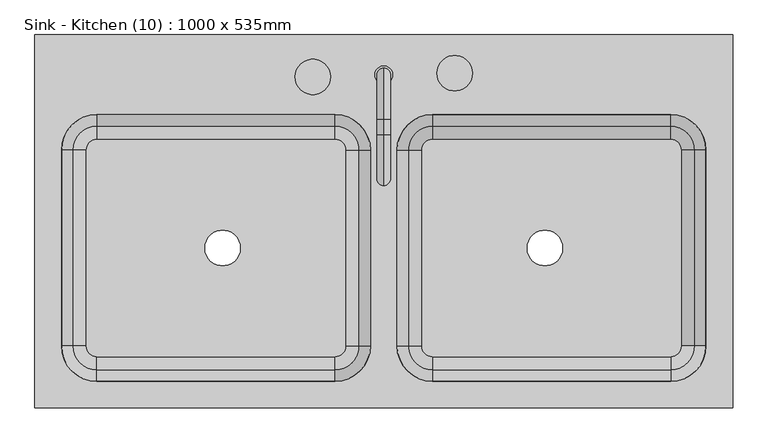
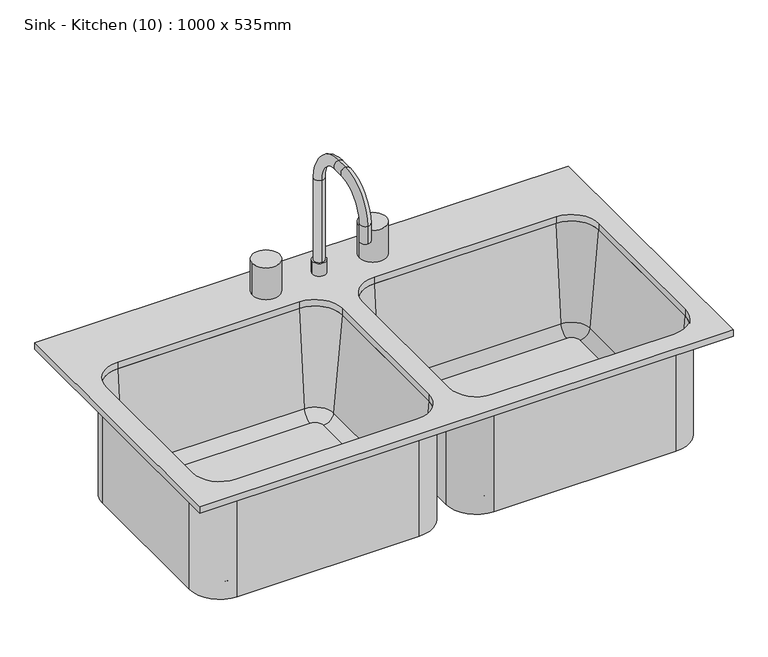
"""IFC4 building model written with IfcOpenShell, lengths in millimetres: flow terminal geometry, Sink - Kitchen (10) : 1000 x 535mm."""

from ifc_helpers import new_model, si_unit, point, frame, frame_2d, origin, place, context, project, spatial, polyline, circle_curve, ellipse_curve, trimmed, segment, composite_curve, outline, extrude, source, transform, mapped, element, save
from ifc_brep_helpers import plane_surface, cylinder_surface, revolved_surface, advanced_brep


def sink_kitchen_10_1000_x_535mm_bc591ed5(model_context):
    return source(origin(), model_context, "Body", "SolidModel", [
        extrude(outline(polyline([(515.6892406, 269.8454011), (515.6892406, -265.1545989), (-484.3107594, -265.1545989), (-484.3107594, 269.8454011), (515.6892406, 269.8454011)]), holes=[composite_curve([segment(polyline([(-54.1607594, 155.5454011), (-395.4107594, 155.5454011)]), True, "CONTINUOUS"), segment(trimmed(circle_curve(frame_2d((-395.4107594, 104.7454011)), 50.8), [point((-395.4107594, 155.5454011))], [point((-446.2107594, 104.7454011))], True, "CARTESIAN"), True, "CONTINUOUS"), segment(polyline([(-446.2107594, 104.7454011), (-446.2107594, -176.2545989)]), True, "CONTINUOUS"), segment(trimmed(circle_curve(frame_2d((-395.4107594, -176.2545989)), 50.8), [point((-446.2107594, -176.2545989))], [point((-395.4107594, -227.0545989))], True, "CARTESIAN"), True, "CONTINUOUS"), segment(polyline([(-395.4107594, -227.0545989), (-54.1607594, -227.0545989)]), True, "CONTINUOUS"), segment(trimmed(circle_curve(frame_2d((-54.1607594, -176.2545989)), 50.8), [point((-54.1607594, -227.0545989))], [point((-3.3607594, -176.2545989))], True, "CARTESIAN"), True, "CONTINUOUS"), segment(polyline([(-3.3607594, -176.2545989), (-3.3607594, 104.7454011)]), True, "CONTINUOUS"), segment(trimmed(circle_curve(frame_2d((-54.1607594, 104.7454011)), 50.8), [point((-3.3607594, 104.7454011))], [point((-54.1607594, 155.5454011))], True, "CARTESIAN"), True, "CONTINUOUS")], self_intersect=False), composite_curve([segment(polyline([(85.5392406, -227.0545989), (426.7892406, -227.0545989)]), True, "CONTINUOUS"), segment(trimmed(circle_curve(frame_2d((426.7892406, -176.2545989)), 50.8), [point((426.7892406, -227.0545989))], [point((477.5892406, -176.2545989))], True, "CARTESIAN"), True, "CONTINUOUS"), segment(polyline([(477.5892406, -176.2545989), (477.5892406, 104.7454011)]), True, "CONTINUOUS"), segment(trimmed(circle_curve(frame_2d((426.7892406, 104.7454011)), 50.8), [point((477.5892406, 104.7454011))], [point((426.7892406, 155.5454011))], True, "CARTESIAN"), True, "CONTINUOUS"), segment(polyline([(426.7892406, 155.5454011), (85.5392406, 155.5454011)]), True, "CONTINUOUS"), segment(trimmed(circle_curve(frame_2d((85.5392406, 104.7454011)), 50.8), [point((85.5392406, 155.5454011))], [point((34.7392406, 104.7454011))], True, "CARTESIAN"), True, "CONTINUOUS"), segment(polyline([(34.7392406, 104.7454011), (34.7392406, -176.2545989)]), True, "CONTINUOUS"), segment(trimmed(circle_curve(frame_2d((85.5392406, -176.2545989)), 50.8), [point((34.7392406, -176.2545989))], [point((85.5392406, -227.0545989))], True, "CARTESIAN"), True, "CONTINUOUS")], self_intersect=False)]), frame((0.0, 0.0, 900.0), z_axis=(0.0, 0.0, 1.0), x_axis=(1.0, 0.0, 0.0)), (0.0, 0.0, 1.0), 12.7),
        extrude(outline(composite_curve([segment(trimmed(circle_curve(frame_2d((-85.9107594, 209.6166076)), 25.4), [point((-111.3107594, 209.6166076))], [point((-60.5107594, 209.6166076))], False, "CARTESIAN"), True, "CONTINUOUS"), segment(trimmed(circle_curve(frame_2d((-85.9107594, 209.6166076)), 25.4), [point((-60.5107594, 209.6166076))], [point((-111.3107594, 209.6166076))], False, "CARTESIAN"), True, "CONTINUOUS")], self_intersect=False)), frame((0.0, 0.0, 912.7), z_axis=(0.0, 0.0, 1.0), x_axis=(1.0, 0.0, 0.0)), (0.0, 0.0, 1.0), 63.5),
        extrude(outline(composite_curve([segment(trimmed(circle_curve(frame_2d((117.2892406, 214.8133323)), 25.4), [point((91.8892406, 214.8133323))], [point((142.6892406, 214.8133323))], False, "CARTESIAN"), True, "CONTINUOUS"), segment(trimmed(circle_curve(frame_2d((117.2892406, 214.8133323)), 25.4), [point((142.6892406, 214.8133323))], [point((91.8892406, 214.8133323))], False, "CARTESIAN"), True, "CONTINUOUS")], self_intersect=False)), frame((0.0, 0.0, 912.7), z_axis=(0.0, 0.0, 1.0), x_axis=(1.0, 0.0, 0.0)), (0.0, 0.0, 1.0), 63.5),
        advanced_brep(
        [(2.9892406, 212.6954011, 912.7), (28.3892406, 212.6954011, 912.7), (15.6892406, 222.2204011, 1100.025), (15.6892406, 203.1704011, 1100.025), (15.6892406, 203.1704011, 938.1), (15.6892406, 222.2204011, 938.1), (15.6892406, 149.1954011, 1173.05), (15.6892406, 149.1954011, 1154.0), (15.6892406, 126.9704011, 1173.05), (15.6892406, 126.9704011, 1154.0), (15.6892406, 53.9454011, 1100.025), (15.6892406, 72.9954011, 1100.025), (15.6892406, 53.9454011, 1065.1), (15.6892406, 72.9954011, 1065.1), (2.9892406, 212.6954011, 938.1), (28.3892406, 212.6954011, 938.1)],
        [
            (0, 1, circle_curve(frame((15.6892406, 212.6954011, 912.7), z_axis=(0.0, 0.0, -1.0), x_axis=(1.0, 0.0, 0.0)), 12.7)),
            (1, 0, circle_curve(frame((15.6892406, 212.6954011, 912.7), z_axis=(0.0, 0.0, -1.0), x_axis=(1.0, 0.0, 0.0)), 12.7)),
            (2, 3, circle_curve(frame((15.6892406, 212.6954011, 1100.025), z_axis=(0.0, 0.0, -1.0), x_axis=(0.0, -1.0, 0.0)), 9.525)),
            (3, 4),
            (4, 5, circle_curve(frame((15.6892406, 212.6954011, 938.1), z_axis=(0.0, 0.0, 1.0), x_axis=(0.0, -1.0, 0.0)), 9.525)),
            (5, 2),
            (3, 2, circle_curve(frame((15.6892406, 212.6954011, 1100.025), z_axis=(0.0, 0.0, -1.0), x_axis=(0.0, -1.0, 0.0)), 9.525)),
            (5, 4, circle_curve(frame((15.6892406, 212.6954011, 938.1), z_axis=(0.0, 0.0, 1.0), x_axis=(0.0, -1.0, 0.0)), 9.525)),
            (2, 6, circle_curve(frame((15.6892406, 149.1954011, 1100.025), z_axis=(1.0, 0.0, 0.0), x_axis=(0.0, 1.0, 0.0)), 73.025)),
            (6, 7, circle_curve(frame((15.6892406, 149.1954011, 1163.525), z_axis=(0.0, 1.0, 0.0), x_axis=(0.0, 0.0, -1.0)), 9.525)),
            (7, 3, circle_curve(frame((15.6892406, 149.1954011, 1100.025), z_axis=(-1.0, 0.0, 0.0), x_axis=(0.0, 1.0, 0.0)), 53.975)),
            (7, 6, circle_curve(frame((15.6892406, 149.1954011, 1163.525), z_axis=(0.0, 1.0, 0.0), x_axis=(0.0, 0.0, -1.0)), 9.525)),
            (6, 8),
            (8, 9, circle_curve(frame((15.6892406, 126.9704011, 1163.525), z_axis=(0.0, 1.0, 0.0), x_axis=(0.0, 0.0, -1.0)), 9.525)),
            (9, 7),
            (9, 8, circle_curve(frame((15.6892406, 126.9704011, 1163.525), z_axis=(0.0, 1.0, 0.0), x_axis=(0.0, 0.0, -1.0)), 9.525)),
            (8, 10, circle_curve(frame((15.6892406, 126.9704011, 1100.025), z_axis=(1.0, 0.0, 0.0), x_axis=(0.0, 0.0, 1.0)), 73.025)),
            (10, 11, circle_curve(frame((15.6892406, 63.4704011, 1100.025), z_axis=(0.0, 0.0, 1.0), x_axis=(0.0, 1.0, 0.0)), 9.525)),
            (11, 9, circle_curve(frame((15.6892406, 126.9704011, 1100.025), z_axis=(-1.0, 0.0, 0.0), x_axis=(0.0, 0.0, 1.0)), 53.975)),
            (11, 10, circle_curve(frame((15.6892406, 63.4704011, 1100.025), z_axis=(0.0, 0.0, 1.0), x_axis=(0.0, 1.0, 0.0)), 9.525)),
            (12, 13, circle_curve(frame((15.6892406, 63.4704011, 1065.1), z_axis=(0.0, 0.0, -1.0), x_axis=(0.0, 1.0, 0.0)), 9.525)),
            (13, 12, circle_curve(frame((15.6892406, 63.4704011, 1065.1), z_axis=(0.0, 0.0, -1.0), x_axis=(0.0, 1.0, 0.0)), 9.525)),
            (10, 12),
            (13, 11),
            (14, 15, circle_curve(frame((15.6892406, 212.6954011, 938.1), z_axis=(0.0, 0.0, 1.0), x_axis=(1.0, 0.0, 0.0)), 12.7)),
            (15, 14, circle_curve(frame((15.6892406, 212.6954011, 938.1), z_axis=(0.0, 0.0, 1.0), x_axis=(1.0, 0.0, 0.0)), 12.7)),
            (14, 0),
            (1, 15),
        ],
        [
            plane_surface(frame((15.6892406, 203.1704011, 912.7), z_axis=(0.0, 0.0, -1.0), x_axis=(1.0, 0.0, 0.0))),
            cylinder_surface(frame((15.6892406, 212.6954011, 912.7), z_axis=(0.0, 0.0, -1.0), x_axis=(0.0, -1.0, 0.0)), 9.525),
            revolved_surface(trimmed(ellipse_curve(frame((15.6892406, 212.6954011, 1100.025), z_axis=(0.0, 0.0, -1.0), x_axis=(0.0, -1.0, 0.0)), 9.525, 9.525), [point((15.6892406, 222.2204011, 1100.025))], [point((15.6892406, 203.1704011, 1100.025))], True, "CARTESIAN"), (15.6892406, 149.1954011, 1100.025), (1.0, 0.0, 0.0)),
            revolved_surface(trimmed(ellipse_curve(frame((15.6892406, 212.6954011, 1100.025), z_axis=(0.0, 0.0, -1.0), x_axis=(0.0, -1.0, 0.0)), 9.525, 9.525), [point((15.6892406, 203.1704011, 1100.025))], [point((15.6892406, 222.2204011, 1100.025))], True, "CARTESIAN"), (15.6892406, 149.1954011, 1100.025), (1.0, 0.0, 0.0)),
            cylinder_surface(frame((15.6892406, 149.1954011, 1163.525), z_axis=(0.0, 1.0, 0.0), x_axis=(0.0, 0.0, -1.0)), 9.525),
            revolved_surface(trimmed(ellipse_curve(frame((15.6892406, 126.9704011, 1163.525), z_axis=(0.0, 1.0, 0.0), x_axis=(0.0, 0.0, -1.0)), 9.525, 9.525), [point((15.6892406, 126.9704011, 1173.05))], [point((15.6892406, 126.9704011, 1154.0))], True, "CARTESIAN"), (15.6892406, 126.9704011, 1100.025), (1.0, 0.0, 0.0)),
            revolved_surface(trimmed(ellipse_curve(frame((15.6892406, 126.9704011, 1163.525), z_axis=(0.0, 1.0, 0.0), x_axis=(0.0, 0.0, -1.0)), 9.525, 9.525), [point((15.6892406, 126.9704011, 1154.0))], [point((15.6892406, 126.9704011, 1173.05))], True, "CARTESIAN"), (15.6892406, 126.9704011, 1100.025), (1.0, 0.0, 0.0)),
            plane_surface(frame((15.6892406, 53.9454011, 1065.1), z_axis=(0.0, 0.0, -1.0), x_axis=(-1.0, 0.0, 0.0))),
            cylinder_surface(frame((15.6892406, 63.4704011, 1100.025), z_axis=(0.0, 0.0, 1.0), x_axis=(0.0, 1.0, 0.0)), 9.525),
            plane_surface(frame((28.3892406, 212.6954011, 938.1), z_axis=(0.0, 0.0, 1.0), x_axis=(0.0, 1.0, 0.0))),
            cylinder_surface(frame((15.6892406, 212.6954011, 912.7), z_axis=(0.0, 0.0, 1.0), x_axis=(1.0, 0.0, 0.0)), 12.7),
        ],
        [
            (0, [[1, 2]]),
            (1, [[3, 4, 5, 6]]),
            (1, [[7, -6, 8, -4]]),
            (2, [[-3, 9, 10, 11]]),
            (3, [[-7, -11, 12, -9]]),
            (4, [[-10, 13, 14, 15]]),
            (4, [[-12, -15, 16, -13]]),
            (5, [[-14, 17, 18, 19]]),
            (6, [[-16, -19, 20, -17]]),
            (7, [[21, 22]]),
            (8, [[-18, 23, -22, 24]]),
            (8, [[-20, -24, -21, -23]]),
            (9, [[25, 26], [-5, -8]]),
            (10, [[-25, 27, -2, 28]]),
            (10, [[-26, -28, -1, -27]]),
        ],
    ),
        advanced_brep(
        [(-38.8723412, 104.7454011, 693.625), (-54.1607594, 120.0338193, 693.625), (-395.4107594, 120.0338193, 693.625), (-410.6991776, 104.7454011, 693.625), (-410.6991776, -176.2545989, 693.625), (-395.4107594, -191.5430171, 693.625), (-54.1607594, -191.5430171, 693.625), (-38.8723412, -176.2545989, 693.625), (-240.6607594, -35.7545989, 693.625), (-189.8607594, -35.7545989, 693.625), (-452.5607594, 104.7454011, 684.1), (-395.4107594, 161.8954011, 684.1), (-54.1607594, 161.8954011, 684.1), (2.9892406, 104.7454011, 684.1), (2.9892406, -176.2545989, 684.1), (-54.1607594, -233.4045989, 684.1), (-395.4107594, -233.4045989, 684.1), (-452.5607594, -176.2545989, 684.1), (-240.6607594, -35.7545989, 684.1), (-189.8607594, -35.7545989, 684.1), (-54.1607594, 161.8954011, 900.0), (2.9892406, 104.7454011, 900.0), (-19.8948322, 104.7454011, 711.0146831), (-54.1607594, 139.0113283, 711.0146831), (-3.3607594, 104.7454011, 900.0), (-54.1607594, 155.5454011, 900.0), (2.9892406, -176.2545989, 900.0), (-19.8948322, -176.2545989, 711.0146831), (-3.3607594, -176.2545989, 900.0), (-54.1607594, -233.4045989, 900.0), (-54.1607594, -210.5205261, 711.0146831), (-54.1607594, -227.0545989, 900.0), (-395.4107594, -233.4045989, 900.0), (-395.4107594, -210.5205261, 711.0146831), (-395.4107594, -227.0545989, 900.0), (-452.5607594, -176.2545989, 900.0), (-429.6766866, -176.2545989, 711.0146831), (-446.2107594, -176.2545989, 900.0), (-452.5607594, 104.7454011, 900.0), (-429.6766866, 104.7454011, 711.0146831), (-446.2107594, 104.7454011, 900.0), (-395.4107594, 161.8954011, 900.0), (-395.4107594, 139.0113283, 711.0146831), (-395.4107594, 155.5454011, 900.0)],
        [
            (0, 1, circle_curve(frame((-54.1607594, 104.7454011, 693.625), z_axis=(0.0, 0.0, 1.0), x_axis=(0.0, 1.0, 0.0)), 15.2884182)),
            (1, 2),
            (2, 3, circle_curve(frame((-395.4107594, 104.7454011, 693.625), z_axis=(0.0, 0.0, 1.0), x_axis=(-1.0, 0.0, 0.0)), 15.2884182)),
            (3, 4),
            (4, 5, circle_curve(frame((-395.4107594, -176.2545989, 693.625), z_axis=(0.0, 0.0, 1.0), x_axis=(0.0, -1.0, 0.0)), 15.2884182)),
            (5, 6),
            (6, 7, circle_curve(frame((-54.1607594, -176.2545989, 693.625), z_axis=(0.0, 0.0, 1.0), x_axis=(1.0, 0.0, 0.0)), 15.2884182)),
            (7, 0),
            (8, 9, circle_curve(frame((-215.2607594, -35.7545989, 693.625), z_axis=(0.0, 0.0, -1.0), x_axis=(1.0, 0.0, 0.0)), 25.4)),
            (9, 8, circle_curve(frame((-215.2607594, -35.7545989, 693.625), z_axis=(0.0, 0.0, -1.0), x_axis=(1.0, 0.0, 0.0)), 25.4)),
            (10, 11, circle_curve(frame((-395.4107594, 104.7454011, 684.1), z_axis=(0.0, 0.0, -1.0), x_axis=(-1.0, 0.0, 0.0)), 57.15)),
            (11, 12),
            (12, 13, circle_curve(frame((-54.1607594, 104.7454011, 684.1), z_axis=(0.0, 0.0, -1.0), x_axis=(0.0, 1.0, 0.0)), 57.15)),
            (13, 14),
            (14, 15, circle_curve(frame((-54.1607594, -176.2545989, 684.1), z_axis=(0.0, 0.0, -1.0), x_axis=(1.0, 0.0, 0.0)), 57.15)),
            (15, 16),
            (16, 17, circle_curve(frame((-395.4107594, -176.2545989, 684.1), z_axis=(0.0, 0.0, -1.0), x_axis=(0.0, -1.0, 0.0)), 57.15)),
            (17, 10),
            (18, 19, circle_curve(frame((-215.2607594, -35.7545989, 684.1), z_axis=(0.0, 0.0, 1.0), x_axis=(1.0, 0.0, 0.0)), 25.4)),
            (19, 18, circle_curve(frame((-215.2607594, -35.7545989, 684.1), z_axis=(0.0, 0.0, 1.0), x_axis=(1.0, 0.0, 0.0)), 25.4)),
            (8, 18),
            (19, 9),
            (12, 20),
            (20, 21, circle_curve(frame((-54.1607594, 104.7454011, 900.0), z_axis=(0.0, 0.0, -1.0), x_axis=(0.0, 1.0, 0.0)), 57.15)),
            (21, 13),
            (0, 22, circle_curve(frame((-38.8723412, 104.7454011, 712.675), z_axis=(0.0, -1.0, 0.0), x_axis=(1.0, 0.0, 0.0)), 19.05)),
            (22, 23, circle_curve(frame((-54.1607594, 104.7454011, 711.0146831), z_axis=(0.0, 0.0, 1.0), x_axis=(0.0, 1.0, 0.0)), 34.2659272)),
            (23, 1, circle_curve(frame((-54.1607594, 120.0338193, 712.675), z_axis=(-1.0, 0.0, 0.0), x_axis=(0.0, 1.0, 0.0)), 19.05)),
            (22, 24),
            (24, 25, circle_curve(frame((-54.1607594, 104.7454011, 900.0), z_axis=(0.0, 0.0, 1.0), x_axis=(0.0, 1.0, 0.0)), 50.8)),
            (25, 23),
            (20, 25),
            (24, 21),
            (21, 26),
            (26, 14),
            (7, 27, circle_curve(frame((-38.8723412, -176.2545989, 712.675), z_axis=(0.0, -1.0, 0.0), x_axis=(1.0, 0.0, 0.0)), 19.05)),
            (27, 22),
            (27, 28),
            (28, 24),
            (28, 26),
            (26, 29, circle_curve(frame((-54.1607594, -176.2545989, 900.0), z_axis=(0.0, 0.0, -1.0), x_axis=(1.0, 0.0, 0.0)), 57.15)),
            (29, 15),
            (6, 30, circle_curve(frame((-54.1607594, -191.5430171, 712.675), z_axis=(-1.0, 0.0, 0.0), x_axis=(0.0, -1.0, 0.0)), 19.05)),
            (30, 27, circle_curve(frame((-54.1607594, -176.2545989, 711.0146831), z_axis=(0.0, 0.0, 1.0), x_axis=(1.0, 0.0, 0.0)), 34.2659272)),
            (30, 31),
            (31, 28, circle_curve(frame((-54.1607594, -176.2545989, 900.0), z_axis=(0.0, 0.0, 1.0), x_axis=(1.0, 0.0, 0.0)), 50.8)),
            (31, 29),
            (29, 32),
            (32, 16),
            (5, 33, circle_curve(frame((-395.4107594, -191.5430171, 712.675), z_axis=(-1.0, 0.0, 0.0), x_axis=(0.0, -1.0, 0.0)), 19.05)),
            (33, 30),
            (33, 34),
            (34, 31),
            (34, 32),
            (32, 35, circle_curve(frame((-395.4107594, -176.2545989, 900.0), z_axis=(0.0, 0.0, -1.0), x_axis=(0.0, -1.0, 0.0)), 57.15)),
            (35, 17),
            (4, 36, circle_curve(frame((-410.6991776, -176.2545989, 712.675), z_axis=(0.0, 1.0, 0.0), x_axis=(-1.0, 0.0, 0.0)), 19.05)),
            (36, 33, circle_curve(frame((-395.4107594, -176.2545989, 711.0146831), z_axis=(0.0, 0.0, 1.0), x_axis=(0.0, -1.0, 0.0)), 34.2659272)),
            (36, 37),
            (37, 34, circle_curve(frame((-395.4107594, -176.2545989, 900.0), z_axis=(0.0, 0.0, 1.0), x_axis=(0.0, -1.0, 0.0)), 50.8)),
            (37, 35),
            (35, 38),
            (38, 10),
            (3, 39, circle_curve(frame((-410.6991776, 104.7454011, 712.675), z_axis=(0.0, 1.0, 0.0), x_axis=(-1.0, 0.0, 0.0)), 19.05)),
            (39, 36),
            (39, 40),
            (40, 37),
            (40, 38),
            (38, 41, circle_curve(frame((-395.4107594, 104.7454011, 900.0), z_axis=(0.0, 0.0, -1.0), x_axis=(-1.0, 0.0, 0.0)), 57.15)),
            (41, 11),
            (2, 42, circle_curve(frame((-395.4107594, 120.0338193, 712.675), z_axis=(1.0, 0.0, 0.0), x_axis=(0.0, 1.0, 0.0)), 19.05)),
            (42, 39, circle_curve(frame((-395.4107594, 104.7454011, 711.0146831), z_axis=(0.0, 0.0, 1.0), x_axis=(-1.0, 0.0, 0.0)), 34.2659272)),
            (42, 43),
            (43, 40, circle_curve(frame((-395.4107594, 104.7454011, 900.0), z_axis=(0.0, 0.0, 1.0), x_axis=(-1.0, 0.0, 0.0)), 50.8)),
            (43, 41),
            (41, 20),
            (23, 42),
            (25, 43),
        ],
        [
            plane_surface(frame((-395.4107594, 117.4454011, 693.625), z_axis=(0.0, 0.0, 1.0), x_axis=(-1.0, 0.0, 0.0))),
            plane_surface(frame((-395.4107594, 117.4454011, 684.1), z_axis=(0.0, 0.0, -1.0), x_axis=(1.0, 0.0, 0.0))),
            revolved_surface(polyline([(-189.8607594, -35.7545989, 684.1), (-189.8607594, -35.7545989, 693.625)]), (-215.2607594, -35.7545989, 0.0), (0.0, 0.0, -1.0)),
            cylinder_surface(frame((-54.1607594, 104.7454011, 0.0), z_axis=(0.0, 0.0, -1.0), x_axis=(0.0, 1.0, 0.0)), 57.15),
            revolved_surface(trimmed(ellipse_curve(frame((-54.1607594, 120.0338193, 712.675), z_axis=(1.0, 0.0, 0.0), x_axis=(0.0, 1.0, 0.0)), 19.05, 19.05), [point((-54.1607594, 120.0338193, 693.625))], [point((-54.1607594, 139.0113283, 711.0146831))], True, "CARTESIAN"), (-54.1607594, 104.7454011, 0.0), (0.0, 0.0, -1.0)),
            revolved_surface(polyline([(-54.1607594, 139.0113283, 711.0146831), (-54.1607594, 155.5454011, 900.0)]), (-54.1607594, 104.7454011, 0.0), (0.0, 0.0, -1.0)),
            plane_surface(frame((-54.1607594, 104.7454011, 900.0), z_axis=(0.0, 0.0, 1.0), x_axis=(0.0, 1.0, 0.0))),
            plane_surface(frame((2.9892406, 104.7454011, 900.0), z_axis=(1.0, 0.0, 0.0), x_axis=(0.0, -1.0, 0.0))),
            revolved_surface(polyline([(-19.8223412, -176.25459890000002, 712.675), (-19.8223412, 104.7454011, 712.675)]), (-38.8723412, 104.7454011, 712.675), (0.0, -1.0, 0.0)),
            plane_surface(frame((-19.8948322, 104.7454011, 711.0146831), z_axis=(-0.9961946980917439, 0.0, 0.08715574274767772), x_axis=(0.0, -1.0, 0.0))),
            plane_surface(frame((-3.3607594, 104.7454011, 900.0), z_axis=(0.0, 0.0, 1.0), x_axis=(0.0, -1.0, 0.0))),
            cylinder_surface(frame((-54.1607594, -176.2545989, 0.0), z_axis=(0.0, 0.0, -1.0), x_axis=(1.0, 0.0, 0.0)), 57.15),
            revolved_surface(trimmed(ellipse_curve(frame((-38.8723412, -176.2545989, 712.675), z_axis=(0.0, -1.0, 0.0), x_axis=(1.0, 0.0, 0.0)), 19.05, 19.05), [point((-38.8723412, -176.2545989, 693.625))], [point((-19.8948322, -176.2545989, 711.0146831))], True, "CARTESIAN"), (-54.1607594, -176.2545989, 0.0), (0.0, 0.0, -1.0)),
            revolved_surface(polyline([(-19.8948322, -176.2545989, 711.0146831), (-3.3607594, -176.2545989, 900.0)]), (-54.1607594, -176.2545989, 0.0), (0.0, 0.0, -1.0)),
            plane_surface(frame((-54.1607594, -176.2545989, 900.0), z_axis=(0.0, 0.0, 1.0), x_axis=(1.0, 0.0, 0.0))),
            plane_surface(frame((-54.1607594, -233.4045989, 900.0), z_axis=(0.0, -1.0, 0.0), x_axis=(-1.0, 0.0, 0.0))),
            revolved_surface(polyline([(-395.4107594, -210.5930171, 712.675), (-54.1607594, -210.5930171, 712.675)]), (-54.1607594, -191.5430171, 712.675), (-1.0, 0.0, 0.0)),
            plane_surface(frame((-54.1607594, -210.5205261, 711.0146831), z_axis=(0.0, 0.9961946980917439, 0.08715574274767772), x_axis=(-1.0, 0.0, 0.0))),
            plane_surface(frame((-54.1607594, -227.0545989, 900.0), z_axis=(0.0, 0.0, 1.0), x_axis=(-1.0, 0.0, 0.0))),
            cylinder_surface(frame((-395.4107594, -176.2545989, 0.0), z_axis=(0.0, 0.0, -1.0), x_axis=(0.0, -1.0, 0.0)), 57.15),
            revolved_surface(trimmed(ellipse_curve(frame((-395.4107594, -191.5430171, 712.675), z_axis=(-1.0, 0.0, 0.0), x_axis=(0.0, -1.0, 0.0)), 19.05, 19.05), [point((-395.4107594, -191.5430171, 693.625))], [point((-395.4107594, -210.5205261, 711.0146831))], True, "CARTESIAN"), (-395.4107594, -176.2545989, 0.0), (0.0, 0.0, -1.0)),
            revolved_surface(polyline([(-395.4107594, -210.5205261, 711.0146831), (-395.4107594, -227.0545989, 900.0)]), (-395.4107594, -176.2545989, 0.0), (0.0, 0.0, -1.0)),
            plane_surface(frame((-395.4107594, -176.2545989, 900.0), z_axis=(0.0, 0.0, 1.0), x_axis=(0.0, -1.0, 0.0))),
            plane_surface(frame((-452.5607594, -176.2545989, 900.0), z_axis=(-1.0, 0.0, 0.0), x_axis=(0.0, 1.0, 0.0))),
            revolved_surface(polyline([(-429.7491776, 104.74540110000001, 712.675), (-429.7491776, -176.2545989, 712.675)]), (-410.6991776, -176.2545989, 712.675), (0.0, 1.0, 0.0)),
            plane_surface(frame((-429.6766866, -176.2545989, 711.0146831), z_axis=(0.9961946980917439, 0.0, 0.08715574274767772), x_axis=(0.0, 1.0, 0.0))),
            plane_surface(frame((-446.2107594, -176.2545989, 900.0), z_axis=(0.0, 0.0, 1.0), x_axis=(0.0, 1.0, 0.0))),
            cylinder_surface(frame((-395.4107594, 104.7454011, 0.0), z_axis=(0.0, 0.0, -1.0), x_axis=(-1.0, 0.0, 0.0)), 57.15),
            revolved_surface(trimmed(ellipse_curve(frame((-410.6991776, 104.7454011, 712.675), z_axis=(0.0, 1.0, 0.0), x_axis=(-1.0, 0.0, 0.0)), 19.05, 19.05), [point((-410.6991776, 104.7454011, 693.625))], [point((-429.6766866, 104.7454011, 711.0146831))], True, "CARTESIAN"), (-395.4107594, 104.7454011, 0.0), (0.0, 0.0, -1.0)),
            revolved_surface(polyline([(-429.6766866, 104.7454011, 711.0146831), (-446.2107594, 104.7454011, 900.0)]), (-395.4107594, 104.7454011, 0.0), (0.0, 0.0, -1.0)),
            plane_surface(frame((-395.4107594, 104.7454011, 900.0), z_axis=(0.0, 0.0, 1.0), x_axis=(-1.0, 0.0, 0.0))),
            plane_surface(frame((-395.4107594, 161.8954011, 900.0), z_axis=(0.0, 1.0, 0.0), x_axis=(1.0, 0.0, 0.0))),
            revolved_surface(polyline([(-54.16075940000002, 139.08381930000002, 712.675), (-395.4107594, 139.08381930000002, 712.675)]), (-395.4107594, 120.0338193, 712.675), (1.0, 0.0, 0.0)),
            plane_surface(frame((-395.4107594, 139.0113283, 711.0146831), z_axis=(0.0, -0.9961946980917439, 0.08715574274767772), x_axis=(1.0, 0.0, 0.0))),
            plane_surface(frame((-395.4107594, 155.5454011, 900.0), z_axis=(0.0, 0.0, 1.0), x_axis=(1.0, 0.0, 0.0))),
        ],
        [
            (0, [[1, 2, 3, 4, 5, 6, 7, 8], [9, 10]]),
            (1, [[11, 12, 13, 14, 15, 16, 17, 18], [19, 20]]),
            (2, [[-9, 21, -20, 22]]),
            (2, [[-10, -22, -19, -21]]),
            (3, [[-13, 23, 24, 25]]),
            (4, [[-1, 26, 27, 28]]),
            (5, [[-27, 29, 30, 31]]),
            (6, [[-24, 32, -30, 33]]),
            (7, [[-25, 34, 35, -14]]),
            (8, [[-26, -8, 36, 37]]),
            (9, [[-29, -37, 38, 39]]),
            (10, [[-33, -39, 40, -34]]),
            (11, [[-35, 41, 42, -15]]),
            (12, [[-36, -7, 43, 44]]),
            (13, [[-38, -44, 45, 46]]),
            (14, [[-40, -46, 47, -41]]),
            (15, [[-42, 48, 49, -16]]),
            (16, [[-43, -6, 50, 51]]),
            (17, [[-45, -51, 52, 53]]),
            (18, [[-47, -53, 54, -48]]),
            (19, [[-49, 55, 56, -17]]),
            (20, [[-50, -5, 57, 58]]),
            (21, [[-52, -58, 59, 60]]),
            (22, [[-54, -60, 61, -55]]),
            (23, [[-56, 62, 63, -18]]),
            (24, [[-57, -4, 64, 65]]),
            (25, [[-59, -65, 66, 67]]),
            (26, [[-61, -67, 68, -62]]),
            (27, [[-63, 69, 70, -11]]),
            (28, [[-64, -3, 71, 72]]),
            (29, [[-66, -72, 73, 74]]),
            (30, [[-68, -74, 75, -69]]),
            (31, [[-23, -12, -70, 76]]),
            (32, [[-28, 77, -71, -2]]),
            (33, [[-31, 78, -73, -77]]),
            (34, [[-32, -76, -75, -78]]),
        ],
    ),
        advanced_brep(
        [(426.7892303, 120.0338193, 693.625), (85.5392406, 120.0338193, 693.625), (70.2508224, 104.7454011, 693.625), (70.2508224, -176.2545989, 693.625), (85.5392406, -191.5430171, 693.625), (426.7892406, -191.5430171, 693.625), (442.0776588, -176.2545989, 693.625), (442.0776588, 104.7454011, 693.625), (221.2392406, -35.7545989, 693.625), (272.0392406, -35.7545989, 693.625), (28.3892406, 104.7454011, 684.1), (85.5392406, 161.8954011, 684.1), (426.7892406, 161.8954011, 684.1), (483.9392406, 104.7454011, 684.1), (483.9392406, -176.2545989, 684.1), (426.7892406, -233.4045989, 684.1), (85.5392406, -233.4045989, 684.1), (28.3892406, -176.2545989, 684.1), (221.2392406, -35.7545989, 684.1), (272.0392406, -35.7545989, 684.1), (34.7392406, 104.7454011, 900.0), (85.5392406, 155.5454011, 900.0), (85.5392406, 161.8954011, 900.0), (28.3892406, 104.7454011, 900.0), (51.2733134, 104.7454011, 711.0146831), (85.5392406, 139.0113283, 711.0146831), (28.3892406, -176.2545989, 900.0), (34.7392406, -176.2545989, 900.0), (51.2733134, -176.2545989, 711.0146831), (85.5392406, -233.4045989, 900.0), (85.5392406, -227.0545989, 900.0), (85.5392406, -210.5205261, 711.0146831), (426.7892406, -233.4045989, 900.0), (426.7892406, -227.0545989, 900.0), (426.7892406, -210.5205261, 711.0146831), (483.9392406, -176.2545989, 900.0), (477.5892406, -176.2545989, 900.0), (461.0551678, -176.2545989, 711.0146831), (483.9392406, 104.7454011, 900.0), (477.5892406, 104.7454011, 900.0), (461.0551678, 104.7454011, 711.0146831), (426.7892406, 161.8954011, 900.0), (426.7892406, 155.5454011, 900.0), (426.7892406, 139.0113283, 711.0146831)],
        [
            (0, 1),
            (1, 2, circle_curve(frame((85.5392406, 104.7454011, 693.625), z_axis=(0.0, 0.0, 1.0), x_axis=(0.0, 1.0, 0.0)), 15.2884182)),
            (2, 3),
            (3, 4, circle_curve(frame((85.5392406, -176.2545989, 693.625), z_axis=(0.0, 0.0, 1.0), x_axis=(-1.0, 0.0, 0.0)), 15.2884182)),
            (4, 5),
            (5, 6, circle_curve(frame((426.7892406, -176.2545989, 693.625), z_axis=(0.0, 0.0, 1.0), x_axis=(0.0, -1.0, 0.0)), 15.2884182)),
            (6, 7),
            (7, 0, circle_curve(frame((426.7892406, 104.7454011, 693.625), z_axis=(0.0, 0.0, 1.0), x_axis=(1.0, 0.0, 0.0)), 15.2884182)),
            (8, 9, circle_curve(frame((246.6392406, -35.7545989, 693.625), z_axis=(0.0, 0.0, -1.0), x_axis=(1.0, 0.0, 0.0)), 25.4)),
            (9, 8, circle_curve(frame((246.6392406, -35.7545989, 693.625), z_axis=(0.0, 0.0, -1.0), x_axis=(1.0, 0.0, 0.0)), 25.4)),
            (10, 11, circle_curve(frame((85.5392406, 104.7454011, 684.1), z_axis=(0.0, 0.0, -1.0), x_axis=(0.0, 1.0, 0.0)), 57.15)),
            (11, 12),
            (12, 13, circle_curve(frame((426.7892406, 104.7454011, 684.1), z_axis=(0.0, 0.0, -1.0), x_axis=(1.0, 0.0, 0.0)), 57.15)),
            (13, 14),
            (14, 15, circle_curve(frame((426.7892406, -176.2545989, 684.1), z_axis=(0.0, 0.0, -1.0), x_axis=(0.0, -1.0, 0.0)), 57.15)),
            (15, 16),
            (16, 17, circle_curve(frame((85.5392406, -176.2545989, 684.1), z_axis=(0.0, 0.0, -1.0), x_axis=(-1.0, 0.0, 0.0)), 57.15)),
            (17, 10),
            (18, 19, circle_curve(frame((246.6392406, -35.7545989, 684.1), z_axis=(0.0, 0.0, 1.0), x_axis=(1.0, 0.0, 0.0)), 25.4)),
            (19, 18, circle_curve(frame((246.6392406, -35.7545989, 684.1), z_axis=(0.0, 0.0, 1.0), x_axis=(1.0, 0.0, 0.0)), 25.4)),
            (8, 18),
            (19, 9),
            (20, 21, circle_curve(frame((85.5392406, 104.7454011, 900.0), z_axis=(0.0, 0.0, -1.0), x_axis=(0.0, 1.0, 0.0)), 50.8)),
            (21, 22),
            (22, 23, circle_curve(frame((85.5392406, 104.7454011, 900.0), z_axis=(0.0, 0.0, 1.0), x_axis=(0.0, 1.0, 0.0)), 57.15)),
            (23, 20),
            (20, 24),
            (24, 25, circle_curve(frame((85.5392406, 104.7454011, 711.0146831), z_axis=(0.0, 0.0, -1.0), x_axis=(0.0, 1.0, 0.0)), 34.2659272)),
            (25, 21),
            (24, 2, circle_curve(frame((70.2508224, 104.7454011, 712.675), z_axis=(0.0, -1.0, 0.0), x_axis=(1.0, 0.0, 0.0)), 19.05)),
            (1, 25, circle_curve(frame((85.5392406, 120.0338193, 712.675), z_axis=(1.0, 0.0, 0.0), x_axis=(0.0, -1.0, 0.0)), 19.05)),
            (22, 11),
            (10, 23),
            (23, 26),
            (26, 27),
            (27, 20),
            (27, 28),
            (28, 24),
            (28, 3, circle_curve(frame((70.2508224, -176.2545989, 712.675), z_axis=(0.0, -1.0, 0.0), x_axis=(1.0, 0.0, 0.0)), 19.05)),
            (17, 26),
            (26, 29, circle_curve(frame((85.5392406, -176.2545989, 900.0), z_axis=(0.0, 0.0, 1.0), x_axis=(-1.0, 0.0, 0.0)), 57.15)),
            (29, 30),
            (30, 27, circle_curve(frame((85.5392406, -176.2545989, 900.0), z_axis=(0.0, 0.0, -1.0), x_axis=(-1.0, 0.0, 0.0)), 50.8)),
            (30, 31),
            (31, 28, circle_curve(frame((85.5392406, -176.2545989, 711.0146831), z_axis=(0.0, 0.0, -1.0), x_axis=(-1.0, 0.0, 0.0)), 34.2659272)),
            (31, 4, circle_curve(frame((85.5392406, -191.5430171, 712.675), z_axis=(1.0, 0.0, 0.0), x_axis=(0.0, 1.0, 0.0)), 19.05)),
            (16, 29),
            (29, 32),
            (32, 33),
            (33, 30),
            (33, 34),
            (34, 31),
            (34, 5, circle_curve(frame((426.7892406, -191.5430171, 712.675), z_axis=(1.0, 0.0, 0.0), x_axis=(0.0, 1.0, 0.0)), 19.05)),
            (15, 32),
            (32, 35, circle_curve(frame((426.7892406, -176.2545989, 900.0), z_axis=(0.0, 0.0, 1.0), x_axis=(0.0, -1.0, 0.0)), 57.15)),
            (35, 36),
            (36, 33, circle_curve(frame((426.7892406, -176.2545989, 900.0), z_axis=(0.0, 0.0, -1.0), x_axis=(0.0, -1.0, 0.0)), 50.8)),
            (36, 37),
            (37, 34, circle_curve(frame((426.7892406, -176.2545989, 711.0146831), z_axis=(0.0, 0.0, -1.0), x_axis=(0.0, -1.0, 0.0)), 34.2659272)),
            (37, 6, circle_curve(frame((442.0776588, -176.2545989, 712.675), z_axis=(0.0, 1.0, 0.0), x_axis=(-1.0, 0.0, 0.0)), 19.05)),
            (14, 35),
            (35, 38),
            (38, 39),
            (39, 36),
            (39, 40),
            (40, 37),
            (40, 7, circle_curve(frame((442.0776588, 104.7454011, 712.675), z_axis=(0.0, 1.0, 0.0), x_axis=(-1.0, 0.0, 0.0)), 19.05)),
            (13, 38),
            (38, 41, circle_curve(frame((426.7892406, 104.7454011, 900.0), z_axis=(0.0, 0.0, 1.0), x_axis=(1.0, 0.0, 0.0)), 57.15)),
            (41, 42),
            (42, 39, circle_curve(frame((426.7892406, 104.7454011, 900.0), z_axis=(0.0, 0.0, -1.0), x_axis=(1.0, 0.0, 0.0)), 50.8)),
            (42, 43),
            (43, 40, circle_curve(frame((426.7892406, 104.7454011, 711.0146831), z_axis=(0.0, 0.0, -1.0), x_axis=(1.0, 0.0, 0.0)), 34.2659272)),
            (43, 0, circle_curve(frame((426.7892406, 120.0338193, 712.675), z_axis=(-1.0, 0.0, 0.0), x_axis=(0.0, -1.0, 0.0)), 19.05)),
            (12, 41),
            (21, 42),
            (41, 22),
            (25, 43),
        ],
        [
            plane_surface(frame((85.5392406, 120.0338193, 693.625), z_axis=(0.0, 0.0, 1.0), x_axis=(-1.0, 0.0, 0.0))),
            plane_surface(frame((85.5392406, 120.0338193, 684.1), z_axis=(0.0, 0.0, -1.0), x_axis=(1.0, 0.0, 0.0))),
            revolved_surface(polyline([(272.03924059999997, -35.7545989, 684.1), (272.03924059999997, -35.7545989, 693.625)]), (246.6392406, -35.7545989, 0.0), (0.0, 0.0, -1.0)),
            plane_surface(frame((85.5392406, 104.7454011, 900.0), z_axis=(0.0, 0.0, 1.0), x_axis=(0.0, 1.0, 0.0))),
            revolved_surface(polyline([(85.5392406, 155.5454011, 900.0), (85.5392406, 139.0113283, 711.0146831)]), (85.5392406, 104.7454011, 0.0), (0.0, 0.0, 1.0)),
            revolved_surface(trimmed(ellipse_curve(frame((85.5392406, 120.0338193, 712.675), z_axis=(-1.0, 0.0, 0.0), x_axis=(0.0, -1.0, 0.0)), 19.05, 19.05), [point((85.5392406, 139.0113283, 711.0146831))], [point((85.5392406, 120.0338193, 693.625))], True, "CARTESIAN"), (85.5392406, 104.7454011, 0.0), (0.0, 0.0, 1.0)),
            cylinder_surface(frame((85.5392406, 104.7454011, 0.0), z_axis=(0.0, 0.0, 1.0), x_axis=(0.0, 1.0, 0.0)), 57.15),
            plane_surface(frame((28.3892406, 104.7454011, 900.0), z_axis=(0.0, 0.0, 1.0), x_axis=(0.0, -1.0, 0.0))),
            plane_surface(frame((34.7392406, 104.7454011, 900.0), z_axis=(0.996194698091745, 0.0, 0.08715574274766558), x_axis=(0.0, -1.0, 0.0))),
            revolved_surface(polyline([(89.3008224, -176.25459890000002, 712.675), (89.3008224, 104.7454011, 712.675)]), (70.2508224, 104.7454011, 712.675), (0.0, -1.0, 0.0)),
            plane_surface(frame((28.3892406, 104.7454011, 684.1), z_axis=(-1.0, 0.0, 0.0), x_axis=(0.0, -1.0, 0.0))),
            plane_surface(frame((85.5392406, -176.2545989, 900.0), z_axis=(0.0, 0.0, 1.0), x_axis=(-1.0, 0.0, 0.0))),
            revolved_surface(polyline([(34.7392406, -176.2545989, 900.0), (51.2733134, -176.2545989, 711.0146831)]), (85.5392406, -176.2545989, 0.0), (0.0, 0.0, 1.0)),
            revolved_surface(trimmed(ellipse_curve(frame((70.2508224, -176.2545989, 712.675), z_axis=(0.0, -1.0, 0.0), x_axis=(1.0, 0.0, 0.0)), 19.05, 19.05), [point((51.2733134, -176.2545989, 711.0146831))], [point((70.2508224, -176.2545989, 693.625))], True, "CARTESIAN"), (85.5392406, -176.2545989, 0.0), (0.0, 0.0, 1.0)),
            cylinder_surface(frame((85.5392406, -176.2545989, 0.0), z_axis=(0.0, 0.0, 1.0), x_axis=(-1.0, 0.0, 0.0)), 57.15),
            plane_surface(frame((85.5392406, -233.4045989, 900.0), z_axis=(0.0, 0.0, 1.0), x_axis=(1.0, 0.0, 0.0))),
            plane_surface(frame((85.5392406, -227.0545989, 900.0), z_axis=(0.0, 0.996194698091745, 0.08715574274766558), x_axis=(1.0, 0.0, 0.0))),
            revolved_surface(polyline([(426.78924059999997, -172.49301709999997, 712.675), (85.5392406, -172.49301709999997, 712.675)]), (85.5392406, -191.5430171, 712.675), (1.0, 0.0, 0.0)),
            plane_surface(frame((85.5392406, -233.4045989, 684.1), z_axis=(0.0, -1.0, 0.0), x_axis=(1.0, 0.0, 0.0))),
            plane_surface(frame((426.7892406, -176.2545989, 900.0), z_axis=(0.0, 0.0, 1.0), x_axis=(0.0, -1.0, 0.0))),
            revolved_surface(polyline([(426.7892406, -227.0545989, 900.0), (426.7892406, -210.5205261, 711.0146831)]), (426.7892406, -176.2545989, 0.0), (0.0, 0.0, 1.0)),
            revolved_surface(trimmed(ellipse_curve(frame((426.7892406, -191.5430171, 712.675), z_axis=(1.0, 0.0, 0.0), x_axis=(0.0, 1.0, 0.0)), 19.05, 19.05), [point((426.7892406, -210.5205261, 711.0146831))], [point((426.7892406, -191.5430171, 693.625))], True, "CARTESIAN"), (426.7892406, -176.2545989, 0.0), (0.0, 0.0, 1.0)),
            cylinder_surface(frame((426.7892406, -176.2545989, 0.0), z_axis=(0.0, 0.0, 1.0), x_axis=(0.0, -1.0, 0.0)), 57.15),
            plane_surface(frame((483.9392406, -176.2545989, 900.0), z_axis=(0.0, 0.0, 1.0), x_axis=(0.0, 1.0, 0.0))),
            plane_surface(frame((477.5892406, -176.2545989, 900.0), z_axis=(-0.996194698091745, 0.0, 0.08715574274766558), x_axis=(0.0, 1.0, 0.0))),
            revolved_surface(polyline([(423.0276588, 104.74540110000001, 712.675), (423.0276588, -176.2545989, 712.675)]), (442.0776588, -176.2545989, 712.675), (0.0, 1.0, 0.0)),
            plane_surface(frame((483.9392406, -176.2545989, 684.1), z_axis=(1.0, 0.0, 0.0), x_axis=(0.0, 1.0, 0.0))),
            plane_surface(frame((426.7892406, 104.7454011, 900.0), z_axis=(0.0, 0.0, 1.0), x_axis=(1.0, 0.0, 0.0))),
            revolved_surface(polyline([(477.5892406, 104.7454011, 900.0), (461.0551678, 104.7454011, 711.0146831)]), (426.7892406, 104.7454011, 0.0), (0.0, 0.0, 1.0)),
            revolved_surface(trimmed(ellipse_curve(frame((442.0776588, 104.7454011, 712.675), z_axis=(0.0, 1.0, 0.0), x_axis=(-1.0, 0.0, 0.0)), 19.05, 19.05), [point((461.0551678, 104.7454011, 711.0146831))], [point((442.0776588, 104.7454011, 693.625))], True, "CARTESIAN"), (426.7892406, 104.7454011, 0.0), (0.0, 0.0, 1.0)),
            cylinder_surface(frame((426.7892406, 104.7454011, 0.0), z_axis=(0.0, 0.0, 1.0), x_axis=(1.0, 0.0, 0.0)), 57.15),
            plane_surface(frame((426.7892406, 161.8954011, 900.0), z_axis=(0.0, 0.0, 1.0), x_axis=(-1.0, 0.0, 0.0))),
            plane_surface(frame((426.7892406, 155.5454011, 900.0), z_axis=(0.0, -0.996194698091745, 0.08715574274766558), x_axis=(-1.0, 0.0, 0.0))),
            revolved_surface(polyline([(85.53924060000003, 100.98381930000001, 712.675), (426.7892406, 100.98381930000001, 712.675)]), (426.7892406, 120.0338193, 712.675), (-1.0, 0.0, 0.0)),
            plane_surface(frame((426.7892406, 161.8954011, 684.1), z_axis=(0.0, 1.0, 0.0), x_axis=(-1.0, 0.0, 0.0))),
        ],
        [
            (0, [[1, 2, 3, 4, 5, 6, 7, 8], [9, 10]]),
            (1, [[11, 12, 13, 14, 15, 16, 17, 18], [19, 20]]),
            (2, [[-9, 21, -20, 22]]),
            (2, [[-10, -22, -19, -21]]),
            (3, [[23, 24, 25, 26]]),
            (4, [[-23, 27, 28, 29]]),
            (5, [[-28, 30, -2, 31]]),
            (6, [[-25, 32, -11, 33]]),
            (7, [[-26, 34, 35, 36]]),
            (8, [[-27, -36, 37, 38]]),
            (9, [[-30, -38, 39, -3]]),
            (10, [[-33, -18, 40, -34]]),
            (11, [[-35, 41, 42, 43]]),
            (12, [[-37, -43, 44, 45]]),
            (13, [[-39, -45, 46, -4]]),
            (14, [[-40, -17, 47, -41]]),
            (15, [[-42, 48, 49, 50]]),
            (16, [[-44, -50, 51, 52]]),
            (17, [[-46, -52, 53, -5]]),
            (18, [[-47, -16, 54, -48]]),
            (19, [[-49, 55, 56, 57]]),
            (20, [[-51, -57, 58, 59]]),
            (21, [[-53, -59, 60, -6]]),
            (22, [[-54, -15, 61, -55]]),
            (23, [[-56, 62, 63, 64]]),
            (24, [[-58, -64, 65, 66]]),
            (25, [[-60, -66, 67, -7]]),
            (26, [[-61, -14, 68, -62]]),
            (27, [[-63, 69, 70, 71]]),
            (28, [[-65, -71, 72, 73]]),
            (29, [[-67, -73, 74, -8]]),
            (30, [[-68, -13, 75, -69]]),
            (31, [[-24, 76, -70, 77]]),
            (32, [[-29, 78, -72, -76]]),
            (33, [[-31, -1, -74, -78]]),
            (34, [[-32, -77, -75, -12]]),
        ],
    ),
    ])


if __name__ == "__main__":
    model = new_model("IFC4")
    model_context = context("Model", 3, world=origin())
    ifc_project = project(units=[si_unit("LENGTHUNIT", "METRE", prefix="MILLI")], contexts=[model_context])
    site = spatial("IfcSite", under=ifc_project)
    building = spatial("IfcBuilding", under=site)
    placement = place(None, origin())
    sink_kitchen_10_1000_x_535mm_shape = sink_kitchen_10_1000_x_535mm_bc591ed5(model_context)
    element("IfcFlowTerminal", 1, ObjectType="Sink - Kitchen (10) : 1000 x 535mm", at=placement, inside=building, context=model_context, shape_type="MappedRepresentation", body=[
        mapped(sink_kitchen_10_1000_x_535mm_shape, transform((0.0, 0.0, 0.0), x_axis=(1.0, 0.0, 0.0), y_axis=(0.0, 1.0, 0.0), z_axis=(0.0, 0.0, 1.0))),
    ])
    save(model, "model.ifc")

# Revit data of these elements
# Type "Sink - Kitchen (10) : 1000 x 535mm"
#   Keynote = "N13/180"
#   Counter Height = 900 mm
#   Depth = 535 mm
#   Width = 1000 mm
#   Fixture Material = Metal - Stainless Steel, Polished
#   Sink Material = Metal - Stainless Steel, Polished
#   Default Elevation = 0
# Element 1 (IfcFlowTerminal, "Sink - Kitchen (10) : 1000 x 535mm")
#   Materials on its faces: "Metal - Stainless Steel, Polished"
# Materials
#   "Metal - Stainless Steel, Polished": class "Metal", colour RGB 247 247 247, transparency 0
